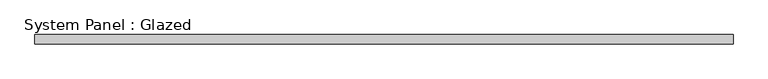
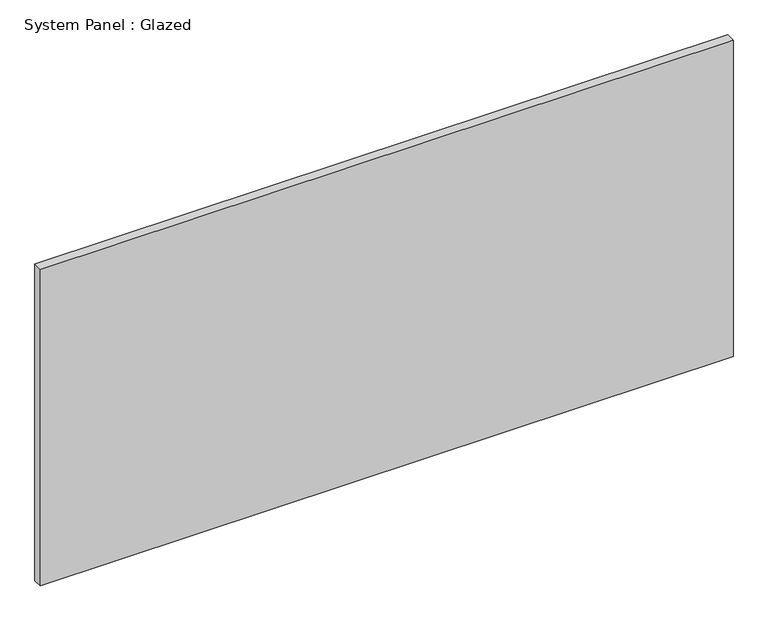
"""IFC4 building model written with IfcOpenShell, lengths in millimetres: plate geometry, System Panel : Glazed."""

from ifc_helpers import new_model, si_unit, origin, origin_with_axes, place, context, project, spatial, polyline, outline, extrude, source, transform, mapped, element, save


def system_panel_glazed_6e11b836(model_context):
    return source(origin(), model_context, "Body", "SweptSolid", [
        extrude(outline(polyline([(951.4416667, 19.05), (-951.4416667, 19.05), (-951.4416667, 44.45), (951.4416667, 44.45), (951.4416667, 19.05)])), origin_with_axes(), (0.0, 0.0, 1.0), 919.5943516),
    ])


if __name__ == "__main__":
    model = new_model("IFC4")
    model_context = context("Model", 3, world=origin())
    ifc_project = project(units=[si_unit("LENGTHUNIT", "METRE", prefix="MILLI")], contexts=[model_context])
    site = spatial("IfcSite", under=ifc_project)
    building = spatial("IfcBuilding", under=site)
    placement = place(None, origin())
    system_panel_glazed_shape = system_panel_glazed_6e11b836(model_context)
    element("IfcPlate", 1, ObjectType="System Panel : Glazed", at=placement, inside=building, context=model_context, shape_type="MappedRepresentation", body=[
        mapped(system_panel_glazed_shape, transform((0.0, 0.0, 0.0), x_axis=(1.0, 0.0, 0.0), y_axis=(0.0, 1.0, 0.0), z_axis=(0.0, 0.0, 1.0))),
    ])
    save(model, "model.ifc")

# Revit data of these elements
# Type "System Panel : Glazed"
#   Construction Type Id = "GSP4R"
#   Analytic Construction = "1/8 in Pilkington single glazing"
#   Visual Light Transmittance = 0.9
#   Solar Heat Gain Coefficient = 0.86
#   Heat Transfer Coefficient (U) = 1.18115 BTU/(h·ft²·°F)
#   Define Thermal Properties by = 1
# Element 1 (IfcPlate, "System Panel : Glazed")
#   Materials on its faces: "Glass"
# Materials
#   "Glass": class "Glass", colour RGB 0 128 192, transparency 0.75, Description = "Soda Lime Glass", Cost = 0
